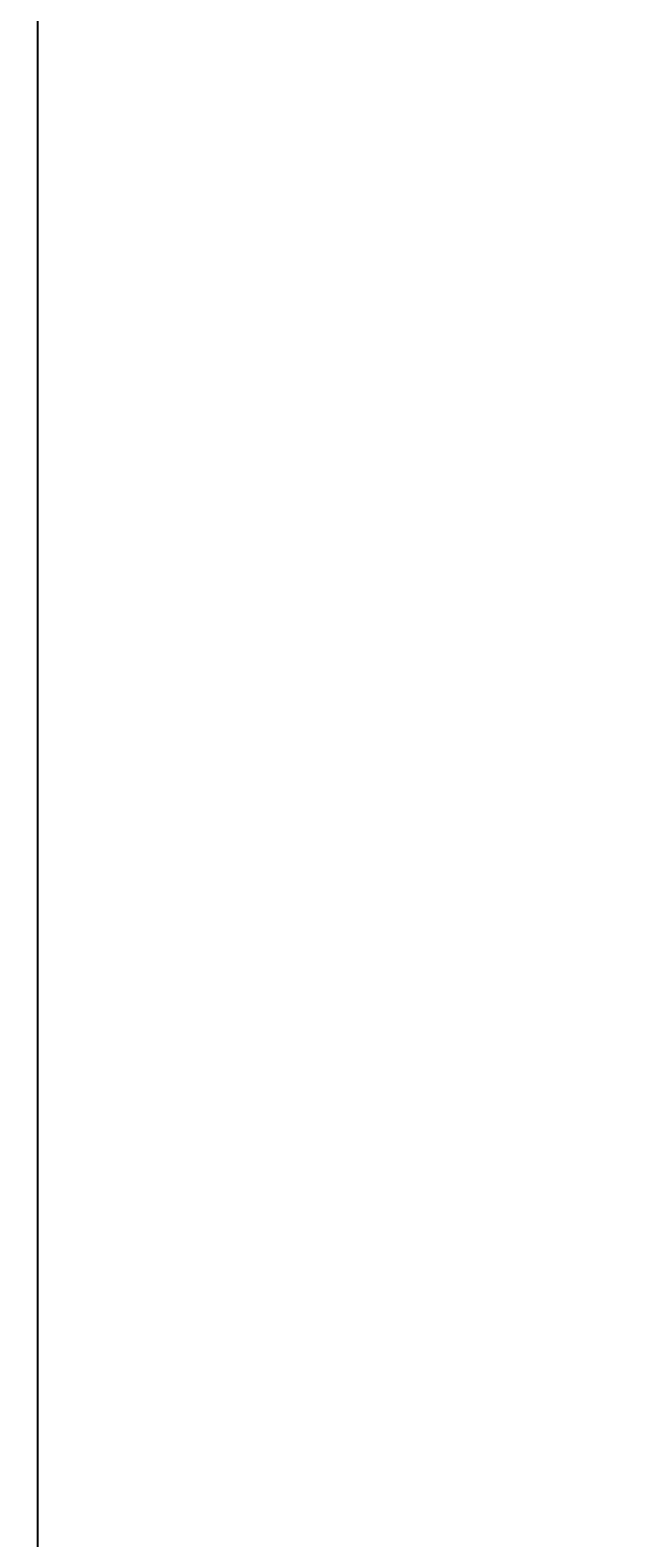
# Model space of a CAD drawing. Units: feet. Extents: x 2695 to 2912, y 795 to 1139.
# Tile 5 of 83: x 2695 to 2710, y 835 to 875. Entities that reach past the tile are written whole.
import ezdxf

# ---------------------------------------------------------------- set-up
doc = ezdxf.new("R2010")
doc.units = ezdxf.units.FT
doc.layers.add('A-ANNO-DIMS', color=2, linetype='Continuous', lineweight=18)
doc.styles.get("Standard").update_dxf_attribs({"font": 'arial.ttf'})
doc.dimstyles.get("Standard").update_dxf_attribs({"dimtxt": 0.18, "dimasz": 0.18, "dimexe": 0.18, "dimexo": 0.0625, "dimgap": 0.09, "dimtad": 0, "dimtih": 1, "dimtoh": 1, "dimdec": 1, "dimzin": 0, "dimdsep": 46, "dimlunit": 3, "dimtxsty": 'Standard', "dimcen": 0.09, "dimadec": 0, "dimazin": 0, "dimtfac": 1, "dimtdec": 1, "dimtofl": 0, "dimtmove": 0, "dimatfit": 3, "dimfxl": 1, "dimtolj": 1, "dimtzin": 0, "dimarcsym": 0})

# ---------------------------------------------------------------- blocks, each defined once
blk = doc.blocks.new('*D12')
at = {"layer": 'A-ANNO-DIMS', "color": 0, "lineweight": -2, "transparency": 16777216}
for p, q in [((2710.574, 1122.931), (2694.681, 1122.931)), ((2694.861, 1122.751), (2694.861, 967.113)), ((2694.861, 811.111), (2694.861, 966.749)), ((2710.574, 810.931), (2694.681, 810.931))]:
    blk.add_line(p, q, dxfattribs=at)
at = {"layer": 'A-ANNO-DIMS', "color": 0, "transparency": 16777216}
for points in [[(2694.831, 1122.751), (2694.891, 1122.751), (2694.861, 1122.931)], [(2694.831, 811.111), (2694.891, 811.111), (2694.861, 810.931)]]:
    blk.add_solid(points, dxfattribs=at)
at = {"layer": 'Defpoints', "color": 0, "transparency": 16777216}
for p in [(2694.861, 1122.931), (2710.636, 1122.931), (2710.636, 810.931)]:
    blk.add_point(p, dxfattribs=at)
at = {"layer": 'A-ANNO-DIMS', "color": 0, "transparency": 16777216, "insert": (2694.861, 966.931), "char_height": 0.18, "attachment_point": 5}
blk.add_mtext('\\A1;312', dxfattribs=at)

msp = doc.modelspace()

# ---------------------------------------------------------------- dimensions: what is measured, and where the dimension line sits
at = {"layer": 'A-ANNO-DIMS'}
dim = msp.add_linear_dim(base=(2694.8611, 1122.9306), p1=(2710.6361, 810.9306), p2=(2710.6361, 1122.9306), angle=90, dimstyle='Standard', override={"dimdec": 0, "dimlfac": 1, "dimrnd": 0, "dimzin": 0, "dimdsep": 46, "dimlunit": 2}, dxfattribs=at)
dim.commit()
dim.dimension.update_dxf_attribs({"geometry": '*D12', "text_midpoint": (2694.8611, 966.9306)})

doc.saveas('drawing.dxf')
